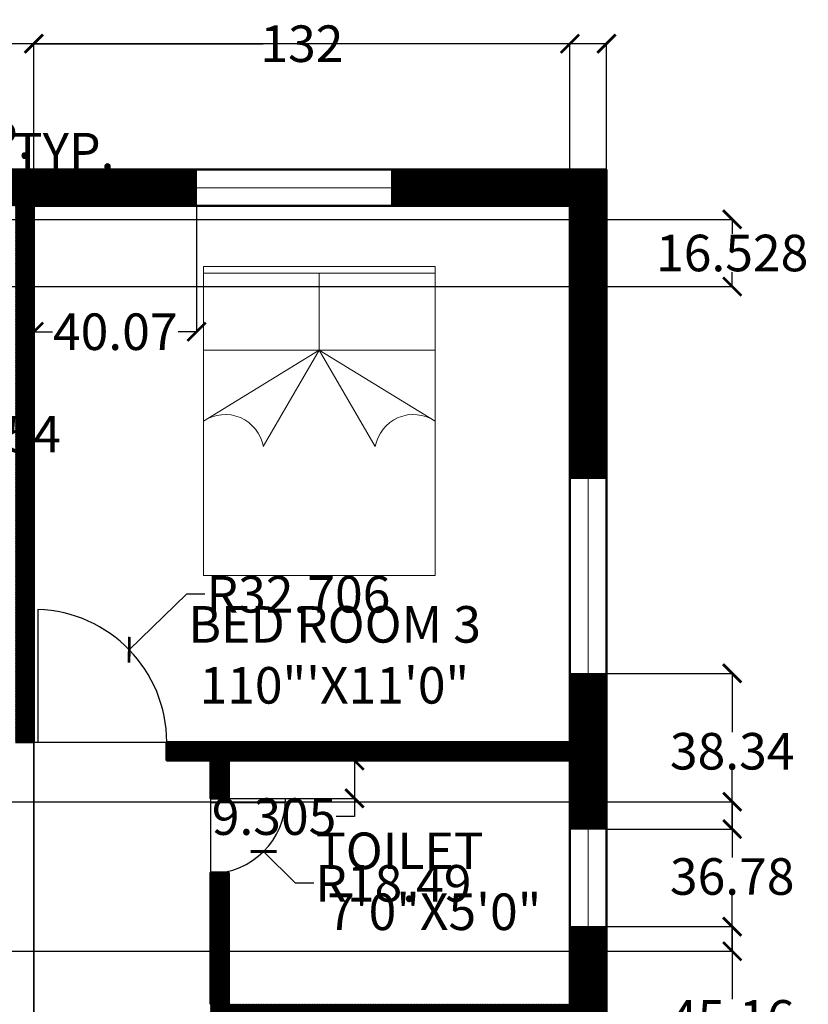
# Model space of a CAD drawing. Units: inches. Extents: x 91 to 526, y 242 to 861.
# Tile 5 of 5: x 332 to 526, y 618 to 861. Entities that reach past the tile are written whole.
import ezdxf

# ---------------------------------------------------------------- set-up
doc = ezdxf.new("R2010")
doc.units = ezdxf.units.IN
doc.header["$MEASUREMENT"] = 0
for name, color, linetype, lineweight in [('A-ANNO-DIMS', 2, 'Continuous', 18), ('A-AREA-IDEN', 7, 'Continuous', 18), ('A-DOOR', 3, 'Continuous', 25), ('A-FURN', 8, 'Continuous', 18), ('A-GLAZ', 4, 'Continuous', 18), ('A-WALL', 7, 'Continuous', 50), ('A-WALL-PATT', 252, 'Continuous', 13)]:
    doc.layers.add(name, color=color, linetype=linetype, lineweight=lineweight)
doc.styles.get("Standard").update_dxf_attribs({"font": 'arial.ttf'})
doc.dimstyles.get("Standard").update_dxf_attribs({"dimtxt": 9, "dimasz": 4.5, "dimexe": 0.18, "dimexo": 0.0625, "dimgap": 0.09, "dimtad": 0, "dimtih": 1, "dimtoh": 1, "dimdec": 1, "dimzin": 0, "dimdsep": 46, "dimlunit": 4, "dimtxsty": 'Standard', "dimblk": 'ARCHTICK', "dimcen": 0.09, "dimadec": 0, "dimazin": 0, "dimtfac": 1, "dimtdec": 1, "dimtofl": 0, "dimtmove": 0, "dimatfit": 3, "dimfxl": 1, "dimtolj": 1, "dimtzin": 0, "dimarcsym": 0})

# ---------------------------------------------------------------- blocks, each defined once
blk = doc.blocks.new('WIN-48')
for p, q in [((0, 9), (48, 9)), ((0, 0), (0, 9)), ((48, 9), (48, 0)), ((0, 4.5), (48, 4.5)), ((48, 0), (0, 0))]:
    blk.add_line(p, q)
blk = doc.blocks.new('WIN-24')
for p, q in [((0, 24), (9, 24)), ((0, 0), (0, 24)), ((4.5, 0), (4.5, 24)), ((9, 24), (9, 0)), ((0, 0), (9, 0))]:
    blk.add_line(p, q)
blk = doc.blocks.new('BED-DOUBLE')
for p, q in [((0, 76.05), (57.04, 76.05)), ((0, 0), (0, 76.05)), ((57.04, 76.05), (57.04, 0)), ((0, 74.47), (57.04, 74.47)), ((28.52, 55.46), (28.52, 74.47)), ((0, 55.46), (57.04, 55.46)), ((28.52, 55.46), (0, 38.03)), ((14.73, 31.74), (28.52, 55.46)), ((57.04, 38.03), (28.52, 55.46)), ((28.52, 55.46), (42.31, 31.74)), ((57.04, 0), (0, 0))]:
    blk.add_line(p, q)
for centre, start, end in [((5.32, 30.09), 9.9572, 123.8152), ((51.72, 30.09), 56.1848, 170.0428)]:
    blk.add_arc(centre, 9.56, start, end)
blk = doc.blocks.new('_ArchTick')
at = {"color": 0, "linetype": 'ByBlock', "const_width": 0.15}
blk.add_lwpolyline([(-0.5, -0.5), (0.5, 0.5)], dxfattribs=at)
blk = doc.blocks.new('*D7')
at = {"layer": 'A-ANNO-DIMS', "color": 0, "lineweight": -2, "transparency": 16777216}
for p, q in [((182.71, 823.73), (182.71, 831.05)), ((182.71, 830.87), (230.71, 830.87)), ((230.71, 823.73), (230.71, 831.05)), ((230.71, 830.87), (235.21, 830.87))]:
    blk.add_line(p, q, dxfattribs=at)
at = {"layer": 'Defpoints', "color": 0, "transparency": 16777216}
for p in [(230.71, 830.87), (182.71, 823.67), (230.71, 823.67)]:
    blk.add_point(p, dxfattribs=at)
at = {"layer": 'A-ANNO-DIMS', "color": 0, "lineweight": -2, "transparency": 16777216, "xscale": 4.5, "yscale": 4.5, "zscale": 4.5, "rotation": 180}
blk.add_blockref('_ArchTick', (182.71, 830.87), dxfattribs=at)
at = {"layer": 'A-ANNO-DIMS', "color": 0, "lineweight": -2, "transparency": 16777216, "xscale": 4.5, "yscale": 4.5, "zscale": 4.5}
blk.add_blockref('_ArchTick', (230.71, 830.87), dxfattribs=at)
at = {"layer": 'A-ANNO-DIMS', "color": 0, "transparency": 16777216, "insert": (286.72, 830.87), "char_height": 9, "attachment_point": 5}
blk.add_mtext('\\A1;WINDOW 48 TYP.', dxfattribs=at)
blk = doc.blocks.new('*D10')
at = {"layer": 'A-ANNO-DIMS', "color": 0, "lineweight": -2, "transparency": 16777216}
for p, q in [((314.7, 823.67), (314.7, 828.17)), ((314.7, 828.17), (319.2, 828.17)), ((311.17, 823.67), (314.88, 823.67)), ((314.7, 814.67), (314.7, 823.67)), ((311.17, 814.67), (314.88, 814.67))]:
    blk.add_line(p, q, dxfattribs=at)
at = {"layer": 'Defpoints', "color": 0, "transparency": 16777216}
for p in [(311.1, 823.67), (314.7, 823.67), (311.1, 814.67)]:
    blk.add_point(p, dxfattribs=at)
at = {"layer": 'A-ANNO-DIMS', "color": 0, "lineweight": -2, "transparency": 16777216, "xscale": 4.5, "yscale": 4.5, "zscale": 4.5}
for p, rotation in [((314.7, 823.67), 90), ((314.7, 814.67), 270)]:
    blk.add_blockref('_ArchTick', p, dxfattribs=dict(at, rotation=rotation))
at = {"layer": 'A-ANNO-DIMS', "color": 0, "transparency": 16777216, "insert": (337.7, 828.17), "char_height": 9, "attachment_point": 5}
blk.add_mtext('\\A1;9 TYP.', dxfattribs=at)
blk = doc.blocks.new('*D17')
at = {"layer": 'A-ANNO-DIMS', "color": 0, "lineweight": -2, "transparency": 16777216}
for p, q in [((137.16, 823.73), (137.16, 854.8)), ((137.16, 854.62), (296.62, 854.62)), ((476.16, 854.62), (316.7, 854.62)), ((476.16, 823.73), (476.16, 854.8))]:
    blk.add_line(p, q, dxfattribs=at)
at = {"layer": 'Defpoints', "color": 0, "transparency": 16777216}
for p in [(476.16, 854.62), (137.16, 823.67), (476.16, 823.67)]:
    blk.add_point(p, dxfattribs=at)
at = {"layer": 'A-ANNO-DIMS', "color": 0, "lineweight": -2, "transparency": 16777216, "xscale": 4.5, "yscale": 4.5, "zscale": 4.5, "rotation": 180}
blk.add_blockref('_ArchTick', (137.16, 854.62), dxfattribs=at)
at = {"layer": 'A-ANNO-DIMS', "color": 0, "lineweight": -2, "transparency": 16777216, "xscale": 4.5, "yscale": 4.5, "zscale": 4.5}
blk.add_blockref('_ArchTick', (476.16, 854.62), dxfattribs=at)
at = {"layer": 'A-ANNO-DIMS', "color": 0, "transparency": 16777216, "insert": (306.66, 854.62), "char_height": 9, "attachment_point": 5}
blk.add_mtext('\\A1;339', dxfattribs=at)
blk = doc.blocks.new('*D21')
at = {"layer": 'A-ANNO-DIMS', "color": 0, "lineweight": -2, "transparency": 16777216}
for p, q in [((335.16, 814.61), (335.16, 783.54)), ((375.23, 814.61), (375.23, 783.54)), ((335.16, 783.72), (339.74, 783.72)), ((375.23, 783.72), (370.65, 783.72))]:
    blk.add_line(p, q, dxfattribs=at)
at = {"layer": 'Defpoints', "color": 0, "transparency": 16777216}
for p in [(335.16, 814.67), (375.23, 814.67), (335.16, 783.72)]:
    blk.add_point(p, dxfattribs=at)
at = {"layer": 'A-ANNO-DIMS', "color": 0, "lineweight": -2, "transparency": 16777216, "xscale": 4.5, "yscale": 4.5, "zscale": 4.5, "rotation": 180}
blk.add_blockref('_ArchTick', (335.16, 783.72), dxfattribs=at)
at = {"layer": 'A-ANNO-DIMS', "color": 0, "lineweight": -2, "transparency": 16777216, "xscale": 4.5, "yscale": 4.5, "zscale": 4.5}
blk.add_blockref('_ArchTick', (375.23, 783.72), dxfattribs=at)
at = {"layer": 'A-ANNO-DIMS', "color": 0, "transparency": 16777216, "insert": (355.2, 783.72), "char_height": 9, "attachment_point": 5}
blk.add_mtext('\\A1;40.07', dxfattribs=at)
blk = doc.blocks.new('*D31')
at = {"layer": 'A-ANNO-DIMS', "color": 0, "lineweight": -2, "transparency": 16777216}
for p, q in [((476.22, 637.29), (507.29, 637.29)), ((507.11, 637.29), (507.11, 619.4)), ((507.11, 592.13), (507.11, 610.03)), ((476.22, 592.13), (507.29, 592.13))]:
    blk.add_line(p, q, dxfattribs=at)
at = {"layer": 'Defpoints', "color": 0, "transparency": 16777216}
for p in [(476.16, 637.29), (507.11, 637.29), (476.16, 592.13)]:
    blk.add_point(p, dxfattribs=at)
at = {"layer": 'A-ANNO-DIMS', "color": 0, "lineweight": -2, "transparency": 16777216, "xscale": 4.5, "yscale": 4.5, "zscale": 4.5}
for p, rotation in [((507.11, 637.29), 90), ((507.11, 592.13), 270)]:
    blk.add_blockref('_ArchTick', p, dxfattribs=dict(at, rotation=rotation))
at = {"layer": 'A-ANNO-DIMS', "color": 0, "transparency": 16777216, "insert": (507.11, 614.71), "char_height": 9, "attachment_point": 5}
blk.add_mtext('\\A1;45.16', dxfattribs=at)
blk = doc.blocks.new('*D32')
at = {"layer": 'A-ANNO-DIMS', "color": 0, "lineweight": -2, "transparency": 16777216}
for p, q in [((476.22, 699.63), (507.29, 699.63)), ((507.11, 699.63), (507.11, 685.15)), ((507.11, 661.29), (507.11, 675.78)), ((476.22, 661.29), (507.29, 661.29))]:
    blk.add_line(p, q, dxfattribs=at)
at = {"layer": 'Defpoints', "color": 0, "transparency": 16777216}
for p in [(476.16, 699.63), (507.11, 699.63), (476.16, 661.29)]:
    blk.add_point(p, dxfattribs=at)
at = {"layer": 'A-ANNO-DIMS', "color": 0, "lineweight": -2, "transparency": 16777216, "xscale": 4.5, "yscale": 4.5, "zscale": 4.5}
for p, rotation in [((507.11, 699.63), 90), ((507.11, 661.29), 270)]:
    blk.add_blockref('_ArchTick', p, dxfattribs=dict(at, rotation=rotation))
at = {"layer": 'A-ANNO-DIMS', "color": 0, "transparency": 16777216, "insert": (507.11, 680.46), "char_height": 9, "attachment_point": 5}
blk.add_mtext('\\A1;38.34', dxfattribs=at)
blk = doc.blocks.new('*D33')
at = {"layer": 'A-ANNO-DIMS', "color": 0, "lineweight": -2, "transparency": 16777216}
for p, q in [((335.16, 814.61), (335.16, 276.54)), ((467.16, 814.61), (467.16, 276.54)), ((335.16, 276.72), (391.6, 276.72)), ((467.16, 276.72), (410.72, 276.72))]:
    blk.add_line(p, q, dxfattribs=at)
at = {"layer": 'Defpoints', "color": 0, "transparency": 16777216}
for p in [(335.16, 814.67), (467.16, 814.67), (467.16, 276.72)]:
    blk.add_point(p, dxfattribs=at)
at = {"layer": 'A-ANNO-DIMS', "color": 0, "lineweight": -2, "transparency": 16777216, "xscale": 4.5, "yscale": 4.5, "zscale": 4.5, "rotation": 180}
blk.add_blockref('_ArchTick', (335.16, 276.72), dxfattribs=at)
at = {"layer": 'A-ANNO-DIMS', "color": 0, "lineweight": -2, "transparency": 16777216, "xscale": 4.5, "yscale": 4.5, "zscale": 4.5}
blk.add_blockref('_ArchTick', (467.16, 276.72), dxfattribs=at)
at = {"layer": 'A-ANNO-DIMS', "color": 0, "transparency": 16777216, "insert": (401.16, 276.72), "char_height": 9, "attachment_point": 5}
blk.add_mtext('\\A1;132', dxfattribs=at)
blk = doc.blocks.new('*D34')
at = {"layer": 'A-ANNO-DIMS', "color": 0, "lineweight": -2, "transparency": 16777216}
for p, q in [((335.16, 316.73), (335.16, 854.8)), ((335.16, 854.62), (391.6, 854.62)), ((467.16, 854.62), (410.72, 854.62)), ((467.16, 316.73), (467.16, 854.8))]:
    blk.add_line(p, q, dxfattribs=at)
at = {"layer": 'Defpoints', "color": 0, "transparency": 16777216}
for p in [(467.16, 854.62), (335.16, 316.67), (467.16, 316.67)]:
    blk.add_point(p, dxfattribs=at)
at = {"layer": 'A-ANNO-DIMS', "color": 0, "lineweight": -2, "transparency": 16777216, "xscale": 4.5, "yscale": 4.5, "zscale": 4.5, "rotation": 180}
blk.add_blockref('_ArchTick', (335.16, 854.62), dxfattribs=at)
at = {"layer": 'A-ANNO-DIMS', "color": 0, "lineweight": -2, "transparency": 16777216, "xscale": 4.5, "yscale": 4.5, "zscale": 4.5}
blk.add_blockref('_ArchTick', (467.16, 854.62), dxfattribs=at)
at = {"layer": 'A-ANNO-DIMS', "color": 0, "transparency": 16777216, "insert": (401.16, 854.62), "char_height": 9, "attachment_point": 5}
blk.add_mtext('\\A1;132', dxfattribs=at)
blk = doc.blocks.new('*D40')
at = {"layer": 'A-ANNO-DIMS', "color": 0, "lineweight": -2, "transparency": 16777216}
for p, q in [((229.85, 811.37), (507.29, 811.37)), ((507.11, 811.37), (507.11, 807.79)), ((507.11, 794.84), (507.11, 798.42)), ((229.85, 794.84), (507.29, 794.84))]:
    blk.add_line(p, q, dxfattribs=at)
at = {"layer": 'Defpoints', "color": 0, "transparency": 16777216}
for p in [(229.79, 811.37), (229.79, 794.84), (507.11, 794.84)]:
    blk.add_point(p, dxfattribs=at)
at = {"layer": 'A-ANNO-DIMS', "color": 0, "lineweight": -2, "transparency": 16777216, "xscale": 4.5, "yscale": 4.5, "zscale": 4.5}
for p, rotation in [((507.11, 811.37), 90), ((507.11, 794.84), 270)]:
    blk.add_blockref('_ArchTick', p, dxfattribs=dict(at, rotation=rotation))
at = {"layer": 'A-ANNO-DIMS', "color": 0, "transparency": 16777216, "insert": (507.11, 803.1), "char_height": 9, "attachment_point": 5}
blk.add_mtext('\\A1;16.528', dxfattribs=at)
blk = doc.blocks.new('*D46')
at = {"layer": 'A-ANNO-DIMS', "color": 0, "lineweight": -2, "transparency": 16777216}
for p, q in [((248.38, 668.02), (507.29, 668.02)), ((507.11, 668.02), (507.11, 654.31)), ((507.11, 631.24), (507.11, 644.94)), ((248.38, 631.24), (507.29, 631.24))]:
    blk.add_line(p, q, dxfattribs=at)
at = {"layer": 'Defpoints', "color": 0, "transparency": 16777216}
for p in [(248.32, 668.02), (507.11, 668.02), (248.32, 631.24)]:
    blk.add_point(p, dxfattribs=at)
at = {"layer": 'A-ANNO-DIMS', "color": 0, "lineweight": -2, "transparency": 16777216, "xscale": 4.5, "yscale": 4.5, "zscale": 4.5}
for p, rotation in [((507.11, 668.02), 90), ((507.11, 631.24), 270)]:
    blk.add_blockref('_ArchTick', p, dxfattribs=dict(at, rotation=rotation))
at = {"layer": 'A-ANNO-DIMS', "color": 0, "transparency": 16777216, "insert": (507.11, 649.63), "char_height": 9, "attachment_point": 5}
blk.add_mtext('\\A1;36.78', dxfattribs=at)
blk = doc.blocks.new('*D53')
at = {"layer": 'A-ANNO-DIMS', "color": 0, "lineweight": -2, "transparency": 16777216}
for p, q in [((383.22, 678.17), (414.29, 678.17)), ((414.11, 678.17), (414.11, 668.87)), ((383.22, 668.87), (414.29, 668.87)), ((414.11, 668.87), (414.11, 664.37)), ((414.11, 664.37), (409.61, 664.37))]:
    blk.add_line(p, q, dxfattribs=at)
at = {"layer": 'Defpoints', "color": 0, "transparency": 16777216}
for p in [(383.16, 678.17), (383.16, 668.87), (414.11, 668.87)]:
    blk.add_point(p, dxfattribs=at)
at = {"layer": 'A-ANNO-DIMS', "color": 0, "lineweight": -2, "transparency": 16777216, "xscale": 4.5, "yscale": 4.5, "zscale": 4.5}
for p, rotation in [((414.11, 678.17), 90), ((414.11, 668.87), 270)]:
    blk.add_blockref('_ArchTick', p, dxfattribs=dict(at, rotation=rotation))
at = {"layer": 'A-ANNO-DIMS', "color": 0, "transparency": 16777216, "insert": (394.3, 664.37), "char_height": 9, "attachment_point": 5}
blk.add_mtext('\\A1;9.305', dxfattribs=at)
blk = doc.blocks.new('*D61')
at = {"layer": 'A-ANNO-DIMS', "color": 0, "lineweight": -2, "transparency": 16777216}
for p, q in [((372.72, 719.1), (358.64, 705.44)), ((377.22, 719.1), (372.72, 719.1)), ((335.07, 682.67), (335.25, 682.67)), ((335.16, 682.58), (335.16, 682.76))]:
    blk.add_line(p, q, dxfattribs=at)
at = {"layer": 'Defpoints', "color": 0, "transparency": 16777216}
for p in [(358.64, 705.44), (335.16, 682.67)]:
    blk.add_point(p, dxfattribs=at)
at = {"layer": 'A-ANNO-DIMS', "color": 0, "lineweight": -2, "transparency": 16777216, "xscale": 4.5, "yscale": 4.5, "zscale": 4.5, "rotation": 224.1242582701353}
blk.add_blockref('_ArchTick', (358.64, 705.44), dxfattribs=at)
at = {"layer": 'A-ANNO-DIMS', "color": 0, "transparency": 16777216, "insert": (400.3, 719.1), "char_height": 9, "attachment_point": 5}
blk.add_mtext('\\A1;R32.706', dxfattribs=at)
blk = doc.blocks.new('*D63')
at = {"layer": 'A-ANNO-DIMS', "color": 0, "lineweight": -2, "transparency": 16777216}
for p, q in [((298.53, 758.5), (286.39, 747.29)), ((303.03, 758.5), (298.53, 758.5)), ((266.07, 728.61), (266.25, 728.61)), ((266.16, 728.52), (266.16, 728.7))]:
    blk.add_line(p, q, dxfattribs=at)
at = {"layer": 'Defpoints', "color": 0, "transparency": 16777216}
for p in [(286.39, 747.29), (266.16, 728.61)]:
    blk.add_point(p, dxfattribs=at)
at = {"layer": 'A-ANNO-DIMS', "color": 0, "lineweight": -2, "transparency": 16777216, "xscale": 4.5, "yscale": 4.5, "zscale": 4.5, "rotation": 222.7186024980729}
blk.add_blockref('_ArchTick', (286.39, 747.29), dxfattribs=at)
at = {"layer": 'A-ANNO-DIMS', "color": 0, "transparency": 16777216, "insert": (322.6, 758.5), "char_height": 9, "attachment_point": 5}
blk.add_mtext('\\A1;R27.54', dxfattribs=at)
blk = doc.blocks.new('*D66')
at = {"layer": 'A-ANNO-DIMS', "color": 0, "lineweight": -2, "transparency": 16777216}
for p, q in [((378.66, 668.78), (378.66, 668.96)), ((378.57, 668.87), (378.75, 668.87)), ((399.58, 647.95), (391.73, 655.79)), ((404.08, 647.95), (399.58, 647.95))]:
    blk.add_line(p, q, dxfattribs=at)
at = {"layer": 'Defpoints', "color": 0, "transparency": 16777216}
for p in [(378.66, 668.87), (391.73, 655.79)]:
    blk.add_point(p, dxfattribs=at)
at = {"layer": 'A-ANNO-DIMS', "color": 0, "lineweight": -2, "transparency": 16777216, "xscale": 4.5, "yscale": 4.5, "zscale": 4.5, "rotation": 134.9998948170958}
blk.add_blockref('_ArchTick', (391.73, 655.79), dxfattribs=at)
at = {"layer": 'A-ANNO-DIMS', "color": 0, "transparency": 16777216, "insert": (423.67, 647.95), "char_height": 9, "attachment_point": 5}
blk.add_mtext('\\A1;R18.49', dxfattribs=at)

msp = doc.modelspace()

# ---------------------------------------------------------------- hatches: boundary and pattern name
at = {"layer": 'A-WALL-PATT'}
h = msp.add_hatch(dxfattribs=at)
h.set_pattern_fill('ANSI31', color=256)
h.paths.add_polyline_path([(476.1605, 544.131), (467.1605, 544.131), (467.1605, 469.6714), (381.2784, 469.6714), (381.2784, 467.1295, -0.01443214), (381.4527, 465.1714), (467.1605, 465.1714), (467.1605, 417.4774), (476.1605, 417.4774)])
h.paths.add_polyline_path([(476.1605, 637.294), (467.1605, 637.294), (467.1605, 618.1714), (383.1605, 618.1714), (383.1605, 650.6481), (381.8098, 650.6481, -0.04281846), (378.6605, 650.378), (378.6605, 618.1714), (378.6605, 613.6714), (467.1605, 613.6714), (467.1605, 592.131), (476.1605, 592.131)])
h.paths.add_polyline_path([(476.1605, 699.6337), (467.1605, 699.6337), (467.1605, 682.6714), (378.6605, 682.6714), (367.8126, 682.6714), (367.8126, 678.1714), (378.6605, 678.1714), (378.6605, 668.8665), (383.1605, 668.8665), (383.1605, 678.1714), (467.1605, 678.1714), (467.1605, 661.294), (476.1605, 661.294)])
h.paths.add_polyline_path([(476.1605, 823.6714), (423.2305, 823.6714), (423.2305, 814.6714), (467.1605, 814.6714), (467.1605, 747.6337), (476.1605, 747.6337)])
h.paths.add_polyline_path([(375.2305, 823.6714), (311.1029, 823.6714), (311.1029, 814.6714), (330.6605, 814.6714), (330.6605, 682.6714), (335.1605, 682.6714), (335.1605, 814.6714), (375.2305, 814.6714)])
h.paths.add_polyline_path([(287.1029, 823.6714), (230.7133, 823.6714), (230.7133, 814.6714), (266.1605, 814.6714), (266.1605, 755.4247), (270.6605, 755.4247), (270.6605, 814.6714), (287.1029, 814.6714)])
h.paths.add_polyline_path([(182.7133, 823.6714), (137.1605, 823.6714), (137.1605, 675.6513), (146.1605, 675.6513), (146.1605, 714.1714), (178.4758, 714.1714), (178.4758, 718.6714), (146.1605, 718.6714), (146.1605, 814.6714), (182.7133, 814.6714)])
h.paths.add_polyline_path([(146.1605, 577.6714), (206.1605, 577.6714), (206.1605, 557.5953), (210.6605, 557.5953), (210.6605, 577.6714), (233.4933, 577.6714), (233.4933, 582.1714), (210.6605, 582.1714), (146.1605, 582.1714), (146.1605, 627.6513), (137.1605, 627.6513), (137.1605, 508.0167), (146.1605, 508.0167), (146.1605, 525.1714), (210.6605, 525.1714), (233.4933, 525.1714), (233.4933, 529.6714), (210.6605, 529.6714), (210.6605, 536.5826), (206.1605, 536.5826), (206.1605, 529.6714), (146.1605, 529.6714)])
h.paths.add_polyline_path([(146.1605, 460.0167), (137.1605, 460.0167), (137.1605, 360.2935), (146.1605, 360.2935), (146.1605, 376.6714), (210.6605, 376.6714), (213.2441, 376.6714, -0.02418169), (213.3544, 378.9513), (213.3544, 381.1714), (210.6605, 381.1714), (146.1605, 381.1714)])
h.paths.add_polyline_path([(146.1605, 336.2935), (137.1605, 336.2935), (137.1605, 307.6714), (146.1605, 307.6714), (177.3362, 307.6714), (177.3362, 316.6714), (146.1605, 316.6714)])
h.paths.add_polyline_path([(393.6086, 316.6714), (323.4726, 316.6714), (323.4726, 307.6714), (393.6086, 307.6714)])
h.paths.add_polyline_path([(256.39, 316.6714), (201.3362, 316.6714), (201.3362, 307.6714), (256.39, 307.6714)])
h.paths.add_polyline_path([(246.6605, 376.6714), (246.6605, 381.1714), (236.8559, 381.1714), (236.8559, 376.6714), (242.1605, 376.6714), (242.1605, 316.6714), (246.6605, 316.6714)])

# ---------------------------------------------------------------- linework, layer by layer
at = {"layer": 'A-DOOR'}
for p, q in [((336.1605, 715.3618), (336.1605, 682.6714)), ((335.1605, 682.6714), (367.8661, 682.6714)), ((378.6605, 668.8665), (397.1491, 668.8665)), ((378.6605, 668.8665), (378.6605, 650.378)), ((378.6605, 667.8665), (397.122, 667.8665))]:
    msp.add_line(p, q, dxfattribs=at)
for centre, radius, start, end in [((335.1605, 682.6714), 32.7056, 0, 88.247864), ((378.6605, 668.8665), 18.4886, 270, 0)]:
    msp.add_arc(centre, radius, start, end, dxfattribs=at)
at = {"layer": 'A-WALL'}
for p, q in [((137.1605, 823.6714), (476.1605, 823.6714)), ((476.1605, 823.6714), (476.1605, 307.6714)), ((335.1605, 814.6714), (335.1605, 682.6714)), ((335.1605, 814.6714), (467.1605, 814.6714)), ((467.1605, 814.6714), (467.1605, 682.6714)), ((335.1605, 682.6714), (330.6605, 682.6714)), ((378.6605, 682.6714), (367.8126, 682.6714)), ((367.8126, 682.6714), (367.8126, 678.1714)), ((378.6605, 682.6714), (467.1605, 682.6714)), ((378.6605, 678.1714), (367.8126, 678.1714)), ((378.6605, 678.1714), (378.6605, 668.8665)), ((383.1605, 678.1714), (467.1605, 678.1714)), ((383.1605, 678.1714), (383.1605, 668.8665)), ((467.1605, 678.1714), (467.1605, 618.1714)), ((378.6605, 668.8665), (383.1605, 668.8665)), ((378.6605, 650.6481), (383.1605, 650.6481)), ((378.6605, 650.6481), (378.6605, 618.1714)), ((383.1605, 650.6481), (383.1605, 618.1714))]:
    msp.add_line(p, q, dxfattribs=at)

# ---------------------------------------------------------------- block references
at = {"layer": 'A-FURN'}
msp.add_blockref('BED-DOUBLE', (376.925, 723.691), dxfattribs=at)
at = {"layer": 'A-GLAZ'}
msp.add_blockref('WIN-48', (375.2302, 814.671), dxfattribs=at)
for name, p, rotation in [('WIN-48', (467.1601, 747.634), 270.0000000000002), ('WIN-24', (476.16, 661.2944), 180)]:
    msp.add_blockref(name, p, dxfattribs=dict(at, rotation=rotation))

# ---------------------------------------------------------------- texts
at = {"layer": 'A-AREA-IDEN', "char_height": 9, "attachment_point": 1}
for s, insert in [('BED ROOM 3\\P 110"\'X11\'0"', (373.2, 716.1906)), ('TOILET\\P 7\'0"X5\'0"', (404.6052, 660.4511))]:
    msp.add_mtext_dynamic_manual_height_columns(s, width=356.121763, gutter_width=1, heights=[0], dxfattribs=dict(at, insert=insert))

# ---------------------------------------------------------------- dimensions: what is measured, and where the dimension line sits
at = {"layer": 'A-ANNO-DIMS'}
for base, p1, p2, picture, middle in [((476.1605, 854.6214), (137.1605, 823.6714), (476.1605, 823.6714), '*D17', (306.6605, 854.6214)), ((467.1605, 854.6214), (335.1605, 316.6714), (467.1605, 316.6714), '*D34', (401.1605, 854.6214)), ((467.1605, 276.7214), (335.1605, 814.6714), (467.1605, 814.6714), '*D33', (401.1605, 276.7214))]:
    dim = msp.add_linear_dim(base=base, p1=p1, p2=p2, dimstyle='Standard', override={"dimdec": 0, "dimlfac": 1, "dimrnd": 0, "dimzin": 0, "dimdsep": 46, "dimlunit": 2}, dxfattribs=at)
    dim.commit()
    dim.dimension.update_dxf_attribs({"geometry": picture, "text_midpoint": middle})
dim = msp.add_linear_dim(base=(230.7133, 830.8714), p1=(182.7133, 823.6714), p2=(230.7133, 823.6714), text='WINDOW <> TYP.', dimstyle='Standard', override={"dimdec": 0, "dimlfac": 1, "dimrnd": 0, "dimzin": 0, "dimdsep": 46, "dimlunit": 2}, dxfattribs=at)
dim.commit()
dim.dimension.update_dxf_attribs({"geometry": '*D7', "text_midpoint": (286.7218, 830.8714)})
dim = msp.add_linear_dim(base=(314.7029, 823.6714), p1=(311.1029, 814.6714), p2=(311.1029, 823.6714), angle=90, text='<> TYP.', dimstyle='Standard', override={"dimdec": 0, "dimlfac": 1, "dimrnd": 0, "dimzin": 0, "dimdsep": 46, "dimlunit": 2}, dxfattribs=at)
dim.commit()
dim.dimension.update_dxf_attribs({"geometry": '*D10', "text_midpoint": (337.7012, 828.1714)})
for base, p1, p2, angle, override, picture, middle in [((335.1605, 783.7214), (375.2305, 814.6714), (335.1605, 814.6714), 180, {"dimdec": 2, "dimlfac": 1, "dimrnd": 0, "dimzin": 0, "dimdsep": 46, "dimlunit": 2}, '*D21', (355.1955, 783.7214)), ((507.1105, 794.8389), (229.7885, 811.367), (229.7885, 794.8389), 90, {"dimdec": 3, "dimlfac": 1, "dimrnd": 0, "dimzin": 0, "dimdsep": 46, "dimlunit": 2}, '*D40', (507.1105, 803.1029)), ((507.1105, 699.6337), (476.1605, 661.294), (476.1605, 699.6337), 90, {"dimdec": 2, "dimlfac": 1, "dimrnd": 0, "dimzin": 0, "dimdsep": 46, "dimlunit": 2}, '*D32', (507.1105, 680.4638)), ((414.1105, 668.8665), (383.1605, 678.1714), (383.1605, 668.8665), 270, {"dimdec": 3, "dimlfac": 1, "dimrnd": 0, "dimzin": 0, "dimdsep": 46, "dimlunit": 2}, '*D53', (394.3015, 664.3665)), ((507.1105, 668.0163), (248.3166, 631.2365), (248.3166, 668.0163), 90, {"dimdec": 2, "dimlfac": 1, "dimrnd": 0, "dimzin": 0, "dimdsep": 46, "dimlunit": 2}, '*D46', (507.1105, 649.6264)), ((507.1105, 637.294), (476.1605, 592.131), (476.1605, 637.294), 90, {"dimdec": 2, "dimlfac": 1, "dimrnd": 0, "dimzin": 0, "dimdsep": 46, "dimlunit": 2}, '*D31', (507.1105, 614.7125))]:
    dim = msp.add_linear_dim(base=base, p1=p1, p2=p2, angle=angle, dimstyle='Standard', override=override, dxfattribs=at)
    dim.commit()
    dim.dimension.update_dxf_attribs({"geometry": picture, "text_midpoint": middle})
for center, mpoint, override, picture, middle in [((266.1605, 728.6069), (286.3938, 747.2898), {"dimdec": 2, "dimlfac": 1, "dimrnd": 0, "dimzin": 0, "dimdsep": 46, "dimlunit": 2}, '*D63', (322.5972, 758.4996)), ((335.1605, 682.6714), (358.6376, 705.4416), {"dimdec": 3, "dimlfac": 1, "dimrnd": 0, "dimzin": 0, "dimdsep": 46, "dimlunit": 2}, '*D61', (400.2989, 719.1038)), ((378.6605, 668.8665), (391.7339, 655.7931), {"dimdec": 2, "dimlfac": 1, "dimrnd": 0, "dimzin": 0, "dimdsep": 46, "dimlunit": 2}, '*D66', (423.6689, 647.9491))]:
    dim = msp.add_radius_dim(center=center, mpoint=mpoint, dimstyle='Standard', override=override, dxfattribs=at)
    dim.commit()
    dim.dimension.update_dxf_attribs({"geometry": picture, "text_midpoint": middle, "dimtype": 164})

doc.saveas('drawing.dxf')
